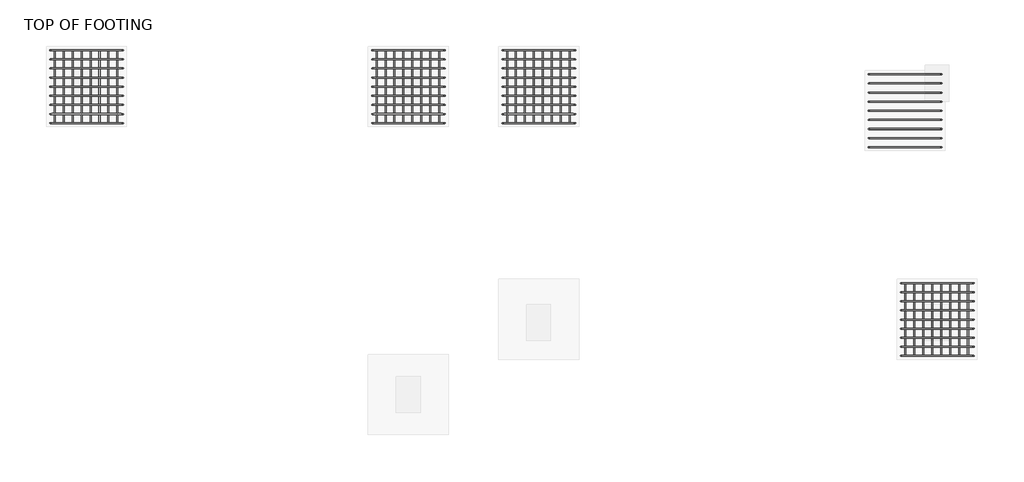
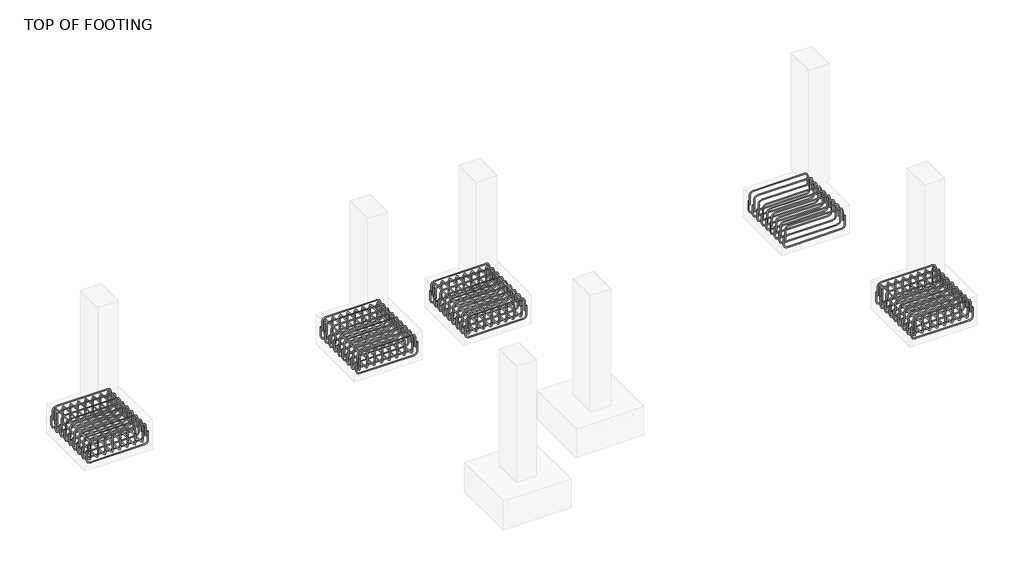
# One storey, part 19 of 20: 18 reinforcing bars.
"""IFC4 building model written with IfcOpenShell, lengths in millimetres."""

from ifc_helpers import new_model, si_unit, point, frame, origin, place, context, project, spatial, polyline, circle_curve, trimmed, segment, composite_curve, source, transform, mapped, element, save
from ifc_brep_helpers import swept_disk

model = new_model("IFC4")

# Units and contexts
model_context = context("Model", 3, world=origin())
ifc_project = project(units=[si_unit("LENGTHUNIT", "METRE", prefix="MILLI")], contexts=[model_context])

# Site, building, storey
site = spatial("IfcSite", under=ifc_project)
building = spatial("IfcBuilding", under=site)
storey = spatial("IfcBuildingStorey", under=building, Name="TOP OF FOOTING", Elevation=-1828.8)

# Reinforcing bars
placement = place(None, origin())
reinforcing_bar_shape = source(origin(), model_context, "Body", "SolidModel", [
    swept_disk(composite_curve([segment(polyline([(2628.3796816, 22141.4849362, -2006.6587682), (2628.3796816, 22141.4849362, -2153.9587682)]), True, "CONTINUOUS"), segment(trimmed(circle_curve(frame((2582.0296816, 22141.4849362, -2153.9587682), z_axis=(0.0, 1.0, 0.0), x_axis=(46.34999999999991, 0.0, 0.0)), 46.35), [point((2628.3796816, 22141.4849362, -2153.9587682))], [point((2582.0296816, 22141.4849362, -2200.3087682))], True, "CARTESIAN"), True, "CONTINUOUS"), segment(polyline([(2582.0296816, 22141.4849362, -2200.3087682), (1767.4296816, 22141.4849362, -2200.3087682)]), True, "CONTINUOUS"), segment(trimmed(circle_curve(frame((1767.4296816, 22141.4849362, -2153.9587682), z_axis=(0.0, 1.0, 0.0), x_axis=(0.0, 0.0, -46.34999999999991)), 46.35), [point((1767.4296816, 22141.4849362, -2200.3087682))], [point((1721.0796816, 22141.4849362, -2153.9587682))], True, "CARTESIAN"), True, "CONTINUOUS"), segment(polyline([(1721.0796816, 22141.4849362, -2153.9587682), (1721.0796816, 22141.4849362, -2006.6587682)]), True, "CONTINUOUS")], self_intersect=False), 6.35),
])
element("IfcReinforcingBar", 1, at=placement, inside=storey, context=model_context, shape_type="MappedRepresentation", body=[
    mapped(reinforcing_bar_shape, transform((0.0, 0.0, 0.0), x_axis=(1.0, 0.0, 0.0), y_axis=(0.0, 1.0, 0.0), z_axis=(0.0, 0.0, 1.0))),
    mapped(reinforcing_bar_shape, transform((0.0, -113.4125, 0.0), x_axis=(1.0, 0.0, 0.0), y_axis=(0.0, 1.0, 0.0), z_axis=(0.0, 0.0, 1.0))),
    mapped(reinforcing_bar_shape, transform((0.0, -226.825, 0.0), x_axis=(1.0, 0.0, 0.0), y_axis=(0.0, 1.0, 0.0), z_axis=(0.0, 0.0, 1.0))),
    mapped(reinforcing_bar_shape, transform((0.0, -340.2375, 0.0), x_axis=(1.0, 0.0, 0.0), y_axis=(0.0, 1.0, 0.0), z_axis=(0.0, 0.0, 1.0))),
    mapped(reinforcing_bar_shape, transform((0.0, -453.65, 0.0), x_axis=(1.0, 0.0, 0.0), y_axis=(0.0, 1.0, 0.0), z_axis=(0.0, 0.0, 1.0))),
    mapped(reinforcing_bar_shape, transform((0.0, -567.0625, 0.0), x_axis=(1.0, 0.0, 0.0), y_axis=(0.0, 1.0, 0.0), z_axis=(0.0, 0.0, 1.0))),
    mapped(reinforcing_bar_shape, transform((0.0, -680.475, 0.0), x_axis=(1.0, 0.0, 0.0), y_axis=(0.0, 1.0, 0.0), z_axis=(0.0, 0.0, 1.0))),
    mapped(reinforcing_bar_shape, transform((0.0, -793.8875, 0.0), x_axis=(1.0, 0.0, 0.0), y_axis=(0.0, 1.0, 0.0), z_axis=(0.0, 0.0, 1.0))),
    mapped(reinforcing_bar_shape, transform((0.0, -907.3, 0.0), x_axis=(1.0, 0.0, 0.0), y_axis=(0.0, 1.0, 0.0), z_axis=(0.0, 0.0, 1.0))),
])
reinforcing_bar_2_shape = source(origin(), model_context, "Body", "SolidModel", [
    swept_disk(composite_curve([segment(polyline([(1740.553793, 22141.4849362, -2068.8), (1740.553793, 22141.4849362, -1921.5)]), True, "CONTINUOUS"), segment(trimmed(circle_curve(frame((1786.903793, 22141.4849362, -1921.5), z_axis=(0.0, 1.0, 0.0), x_axis=(-46.34999999999991, 0.0, 0.0)), 46.35), [point((1740.553793, 22141.4849362, -1921.5))], [point((1786.903793, 22141.4849362, -1875.15))], True, "CARTESIAN"), True, "CONTINUOUS"), segment(polyline([(1786.903793, 22141.4849362, -1875.15), (2556.3671926, 22141.4849362, -1875.15)]), True, "CONTINUOUS"), segment(trimmed(circle_curve(frame((2556.3671926, 22141.4849362, -1921.5), z_axis=(0.0, 1.0, 0.0), x_axis=(0.0, 0.0, 46.34999999999991)), 46.35), [point((2556.3671926, 22141.4849362, -1875.15))], [point((2602.7171926, 22141.4849362, -1921.5))], True, "CARTESIAN"), True, "CONTINUOUS"), segment(polyline([(2602.7171926, 22141.4849362, -1921.5), (2602.7171926, 22141.4849362, -2068.8)]), True, "CONTINUOUS")], self_intersect=False), 6.35),
])
element("IfcReinforcingBar", 2, at=placement, inside=storey, context=model_context, shape_type="MappedRepresentation", body=[
    mapped(reinforcing_bar_2_shape, transform((0.0, 0.0, 0.0), x_axis=(1.0, 0.0, 0.0), y_axis=(0.0, 1.0, 0.0), z_axis=(0.0, 0.0, 1.0))),
    mapped(reinforcing_bar_2_shape, transform((0.0, -113.4125, 0.0), x_axis=(1.0, 0.0, 0.0), y_axis=(0.0, 1.0, 0.0), z_axis=(0.0, 0.0, 1.0))),
    mapped(reinforcing_bar_2_shape, transform((0.0, -226.825, 0.0), x_axis=(1.0, 0.0, 0.0), y_axis=(0.0, 1.0, 0.0), z_axis=(0.0, 0.0, 1.0))),
    mapped(reinforcing_bar_2_shape, transform((0.0, -340.2375, 0.0), x_axis=(1.0, 0.0, 0.0), y_axis=(0.0, 1.0, 0.0), z_axis=(0.0, 0.0, 1.0))),
    mapped(reinforcing_bar_2_shape, transform((0.0, -453.65, 0.0), x_axis=(1.0, 0.0, 0.0), y_axis=(0.0, 1.0, 0.0), z_axis=(0.0, 0.0, 1.0))),
    mapped(reinforcing_bar_2_shape, transform((0.0, -567.0625, 0.0), x_axis=(1.0, 0.0, 0.0), y_axis=(0.0, 1.0, 0.0), z_axis=(0.0, 0.0, 1.0))),
    mapped(reinforcing_bar_2_shape, transform((0.0, -680.475, 0.0), x_axis=(1.0, 0.0, 0.0), y_axis=(0.0, 1.0, 0.0), z_axis=(0.0, 0.0, 1.0))),
    mapped(reinforcing_bar_2_shape, transform((0.0, -793.8875, 0.0), x_axis=(1.0, 0.0, 0.0), y_axis=(0.0, 1.0, 0.0), z_axis=(0.0, 0.0, 1.0))),
    mapped(reinforcing_bar_2_shape, transform((0.0, -907.3, 0.0), x_axis=(1.0, 0.0, 0.0), y_axis=(0.0, 1.0, 0.0), z_axis=(0.0, 0.0, 1.0))),
])
reinforcing_bar_3_shape = source(origin(), model_context, "Body", "SolidModel", [
    swept_disk(composite_curve([segment(polyline([(2556.8827202, 22141.4849362, -2086.1951968), (2556.8827202, 22141.4849362, -1938.8951968)]), True, "CONTINUOUS"), segment(trimmed(circle_curve(frame((2556.8827202, 22095.1349362, -1938.8951968), z_axis=(1.0, 0.0, 0.0), x_axis=(0.0, 46.349999999998545, 0.0)), 46.35), [point((2556.8827202, 22141.4849362, -1938.8951968))], [point((2556.8827202, 22095.1349362, -1892.5451968))], True, "CARTESIAN"), True, "CONTINUOUS"), segment(polyline([(2556.8827202, 22095.1349362, -1892.5451968), (2556.8827202, 21280.5349362, -1892.5451968)]), True, "CONTINUOUS"), segment(trimmed(circle_curve(frame((2556.8827202, 21280.5349362, -1938.8951968), z_axis=(1.0, 0.0, 0.0), x_axis=(0.0, 0.0, 46.34999999999991)), 46.35), [point((2556.8827202, 21280.5349362, -1892.5451968))], [point((2556.8827202, 21234.1849362, -1938.8951968))], True, "CARTESIAN"), True, "CONTINUOUS"), segment(polyline([(2556.8827202, 21234.1849362, -1938.8951968), (2556.8827202, 21234.1849362, -2086.1951968)]), True, "CONTINUOUS")], self_intersect=False), 6.35),
])
element("IfcReinforcingBar", 3, at=placement, inside=storey, context=model_context, shape_type="MappedRepresentation", body=[
    mapped(reinforcing_bar_3_shape, transform((0.0, 0.0, 0.0), x_axis=(1.0, 0.0, 0.0), y_axis=(0.0, 1.0, 0.0), z_axis=(0.0, 0.0, 1.0))),
    mapped(reinforcing_bar_3_shape, transform((-111.2862402, 0.0, 0.0), x_axis=(1.0, 0.0, 0.0), y_axis=(0.0, 1.0, 0.0), z_axis=(0.0, 0.0, 1.0))),
    mapped(reinforcing_bar_3_shape, transform((-222.5724804, 0.0, 0.0), x_axis=(1.0, 0.0, 0.0), y_axis=(0.0, 1.0, 0.0), z_axis=(0.0, 0.0, 1.0))),
    mapped(reinforcing_bar_3_shape, transform((-333.8587205, 0.0, 0.0), x_axis=(1.0, 0.0, 0.0), y_axis=(0.0, 1.0, 0.0), z_axis=(0.0, 0.0, 1.0))),
    mapped(reinforcing_bar_3_shape, transform((-445.1449607, 0.0, 0.0), x_axis=(1.0, 0.0, 0.0), y_axis=(0.0, 1.0, 0.0), z_axis=(0.0, 0.0, 1.0))),
    mapped(reinforcing_bar_3_shape, transform((-556.4312009, 0.0, 0.0), x_axis=(1.0, 0.0, 0.0), y_axis=(0.0, 1.0, 0.0), z_axis=(0.0, 0.0, 1.0))),
    mapped(reinforcing_bar_3_shape, transform((-667.7174411, 0.0, 0.0), x_axis=(1.0, 0.0, 0.0), y_axis=(0.0, 1.0, 0.0), z_axis=(0.0, 0.0, 1.0))),
    mapped(reinforcing_bar_3_shape, transform((-779.0036813, 0.0, 0.0), x_axis=(1.0, 0.0, 0.0), y_axis=(0.0, 1.0, 0.0), z_axis=(0.0, 0.0, 1.0))),
])
reinforcing_bar_4_shape = source(origin(), model_context, "Body", "SolidModel", [
    swept_disk(composite_curve([segment(polyline([(1777.879039, 22141.4849362, -1979.1645013), (1777.879039, 22141.4849362, -2126.4645013)]), True, "CONTINUOUS"), segment(trimmed(circle_curve(frame((1777.879039, 22095.1349362, -2126.4645013), z_axis=(-1.0, 0.0, 0.0), x_axis=(0.0, 46.349999999998545, 0.0)), 46.35), [point((1777.879039, 22141.4849362, -2126.4645013))], [point((1777.879039, 22095.1349362, -2172.8145013))], True, "CARTESIAN"), True, "CONTINUOUS"), segment(polyline([(1777.879039, 22095.1349362, -2172.8145013), (1777.879039, 21280.5349362, -2172.8145013)]), True, "CONTINUOUS"), segment(trimmed(circle_curve(frame((1777.879039, 21280.5349362, -2126.4645013), z_axis=(-1.0, 0.0, 0.0), x_axis=(0.0, 0.0, -46.34999999999991)), 46.35), [point((1777.879039, 21280.5349362, -2172.8145013))], [point((1777.879039, 21234.1849362, -2126.4645013))], True, "CARTESIAN"), True, "CONTINUOUS"), segment(polyline([(1777.879039, 21234.1849362, -2126.4645013), (1777.879039, 21234.1849362, -1979.1645013)]), True, "CONTINUOUS")], self_intersect=False), 6.35),
])
element("IfcReinforcingBar", 4, at=placement, inside=storey, context=model_context, shape_type="MappedRepresentation", body=[
    mapped(reinforcing_bar_4_shape, transform((0.0, 0.0, 0.0), x_axis=(1.0, 0.0, 0.0), y_axis=(0.0, 1.0, 0.0), z_axis=(0.0, 0.0, 1.0))),
    mapped(reinforcing_bar_4_shape, transform((111.2862402, 0.0, 0.0), x_axis=(1.0, 0.0, 0.0), y_axis=(0.0, 1.0, 0.0), z_axis=(0.0, 0.0, 1.0))),
    mapped(reinforcing_bar_4_shape, transform((222.5724804, 0.0, 0.0), x_axis=(1.0, 0.0, 0.0), y_axis=(0.0, 1.0, 0.0), z_axis=(0.0, 0.0, 1.0))),
    mapped(reinforcing_bar_4_shape, transform((333.8587205, 0.0, 0.0), x_axis=(1.0, 0.0, 0.0), y_axis=(0.0, 1.0, 0.0), z_axis=(0.0, 0.0, 1.0))),
    mapped(reinforcing_bar_4_shape, transform((445.1449607, 0.0, 0.0), x_axis=(1.0, 0.0, 0.0), y_axis=(0.0, 1.0, 0.0), z_axis=(0.0, 0.0, 1.0))),
    mapped(reinforcing_bar_4_shape, transform((556.4312009, 0.0, 0.0), x_axis=(1.0, 0.0, 0.0), y_axis=(0.0, 1.0, 0.0), z_axis=(0.0, 0.0, 1.0))),
    mapped(reinforcing_bar_4_shape, transform((667.7174411, 0.0, 0.0), x_axis=(1.0, 0.0, 0.0), y_axis=(0.0, 1.0, 0.0), z_axis=(0.0, 0.0, 1.0))),
    mapped(reinforcing_bar_4_shape, transform((779.0036813, 0.0, 0.0), x_axis=(1.0, 0.0, 0.0), y_axis=(0.0, 1.0, 0.0), z_axis=(0.0, 0.0, 1.0))),
])
reinforcing_bar_5_shape = source(origin(), model_context, "Body", "SolidModel", [
    swept_disk(composite_curve([segment(polyline([(6636.1748054, 22141.4849362, -2006.6587682), (6636.1748054, 22141.4849362, -2153.9587682)]), True, "CONTINUOUS"), segment(trimmed(circle_curve(frame((6589.8248054, 22141.4849362, -2153.9587682), z_axis=(0.0, 1.0, 0.0), x_axis=(46.350000000000364, 0.0, 0.0)), 46.35), [point((6636.1748054, 22141.4849362, -2153.9587682))], [point((6589.8248054, 22141.4849362, -2200.3087682))], True, "CARTESIAN"), True, "CONTINUOUS"), segment(polyline([(6589.8248054, 22141.4849362, -2200.3087682), (5775.2248054, 22141.4849362, -2200.3087682)]), True, "CONTINUOUS"), segment(trimmed(circle_curve(frame((5775.2248054, 22141.4849362, -2153.9587682), z_axis=(0.0, 1.0, 0.0), x_axis=(0.0, 0.0, -46.34999999999991)), 46.35), [point((5775.2248054, 22141.4849362, -2200.3087682))], [point((5728.8748054, 22141.4849362, -2153.9587682))], True, "CARTESIAN"), True, "CONTINUOUS"), segment(polyline([(5728.8748054, 22141.4849362, -2153.9587682), (5728.8748054, 22141.4849362, -2006.6587682)]), True, "CONTINUOUS")], self_intersect=False), 6.35),
])
element("IfcReinforcingBar", 5, at=placement, inside=storey, context=model_context, shape_type="MappedRepresentation", body=[
    mapped(reinforcing_bar_5_shape, transform((0.0, 0.0, 0.0), x_axis=(1.0, 0.0, 0.0), y_axis=(0.0, 1.0, 0.0), z_axis=(0.0, 0.0, 1.0))),
    mapped(reinforcing_bar_5_shape, transform((0.0, -113.4125, 0.0), x_axis=(1.0, 0.0, 0.0), y_axis=(0.0, 1.0, 0.0), z_axis=(0.0, 0.0, 1.0))),
    mapped(reinforcing_bar_5_shape, transform((0.0, -226.825, 0.0), x_axis=(1.0, 0.0, 0.0), y_axis=(0.0, 1.0, 0.0), z_axis=(0.0, 0.0, 1.0))),
    mapped(reinforcing_bar_5_shape, transform((0.0, -340.2375, 0.0), x_axis=(1.0, 0.0, 0.0), y_axis=(0.0, 1.0, 0.0), z_axis=(0.0, 0.0, 1.0))),
    mapped(reinforcing_bar_5_shape, transform((0.0, -453.65, 0.0), x_axis=(1.0, 0.0, 0.0), y_axis=(0.0, 1.0, 0.0), z_axis=(0.0, 0.0, 1.0))),
    mapped(reinforcing_bar_5_shape, transform((0.0, -567.0625, 0.0), x_axis=(1.0, 0.0, 0.0), y_axis=(0.0, 1.0, 0.0), z_axis=(0.0, 0.0, 1.0))),
    mapped(reinforcing_bar_5_shape, transform((0.0, -680.475, 0.0), x_axis=(1.0, 0.0, 0.0), y_axis=(0.0, 1.0, 0.0), z_axis=(0.0, 0.0, 1.0))),
    mapped(reinforcing_bar_5_shape, transform((0.0, -793.8875, 0.0), x_axis=(1.0, 0.0, 0.0), y_axis=(0.0, 1.0, 0.0), z_axis=(0.0, 0.0, 1.0))),
    mapped(reinforcing_bar_5_shape, transform((0.0, -907.3, 0.0), x_axis=(1.0, 0.0, 0.0), y_axis=(0.0, 1.0, 0.0), z_axis=(0.0, 0.0, 1.0))),
])
reinforcing_bar_6_shape = source(origin(), model_context, "Body", "SolidModel", [
    swept_disk(composite_curve([segment(polyline([(5748.3489167, 22141.4849362, -2068.8), (5748.3489167, 22141.4849362, -1921.5)]), True, "CONTINUOUS"), segment(trimmed(circle_curve(frame((5794.6989167, 22141.4849362, -1921.5), z_axis=(0.0, 1.0, 0.0), x_axis=(-46.350000000000364, 0.0, 0.0)), 46.35), [point((5748.3489167, 22141.4849362, -1921.5))], [point((5794.6989167, 22141.4849362, -1875.15))], True, "CARTESIAN"), True, "CONTINUOUS"), segment(polyline([(5794.6989167, 22141.4849362, -1875.15), (6564.1623164, 22141.4849362, -1875.15)]), True, "CONTINUOUS"), segment(trimmed(circle_curve(frame((6564.1623164, 22141.4849362, -1921.5), z_axis=(0.0, 1.0, 0.0), x_axis=(0.0, 0.0, 46.34999999999991)), 46.35), [point((6564.1623164, 22141.4849362, -1875.15))], [point((6610.5123164, 22141.4849362, -1921.5))], True, "CARTESIAN"), True, "CONTINUOUS"), segment(polyline([(6610.5123164, 22141.4849362, -1921.5), (6610.5123164, 22141.4849362, -2068.8)]), True, "CONTINUOUS")], self_intersect=False), 6.35),
])
element("IfcReinforcingBar", 6, at=placement, inside=storey, context=model_context, shape_type="MappedRepresentation", body=[
    mapped(reinforcing_bar_6_shape, transform((0.0, 0.0, 0.0), x_axis=(1.0, 0.0, 0.0), y_axis=(0.0, 1.0, 0.0), z_axis=(0.0, 0.0, 1.0))),
    mapped(reinforcing_bar_6_shape, transform((0.0, -113.4125, 0.0), x_axis=(1.0, 0.0, 0.0), y_axis=(0.0, 1.0, 0.0), z_axis=(0.0, 0.0, 1.0))),
    mapped(reinforcing_bar_6_shape, transform((0.0, -226.825, 0.0), x_axis=(1.0, 0.0, 0.0), y_axis=(0.0, 1.0, 0.0), z_axis=(0.0, 0.0, 1.0))),
    mapped(reinforcing_bar_6_shape, transform((0.0, -340.2375, 0.0), x_axis=(1.0, 0.0, 0.0), y_axis=(0.0, 1.0, 0.0), z_axis=(0.0, 0.0, 1.0))),
    mapped(reinforcing_bar_6_shape, transform((0.0, -453.65, 0.0), x_axis=(1.0, 0.0, 0.0), y_axis=(0.0, 1.0, 0.0), z_axis=(0.0, 0.0, 1.0))),
    mapped(reinforcing_bar_6_shape, transform((0.0, -567.0625, 0.0), x_axis=(1.0, 0.0, 0.0), y_axis=(0.0, 1.0, 0.0), z_axis=(0.0, 0.0, 1.0))),
    mapped(reinforcing_bar_6_shape, transform((0.0, -680.475, 0.0), x_axis=(1.0, 0.0, 0.0), y_axis=(0.0, 1.0, 0.0), z_axis=(0.0, 0.0, 1.0))),
    mapped(reinforcing_bar_6_shape, transform((0.0, -793.8875, 0.0), x_axis=(1.0, 0.0, 0.0), y_axis=(0.0, 1.0, 0.0), z_axis=(0.0, 0.0, 1.0))),
    mapped(reinforcing_bar_6_shape, transform((0.0, -907.3, 0.0), x_axis=(1.0, 0.0, 0.0), y_axis=(0.0, 1.0, 0.0), z_axis=(0.0, 0.0, 1.0))),
])
reinforcing_bar_7_shape = source(origin(), model_context, "Body", "SolidModel", [
    swept_disk(composite_curve([segment(polyline([(6564.677844, 22141.4849362, -2086.1951968), (6564.677844, 22141.4849362, -1938.8951968)]), True, "CONTINUOUS"), segment(trimmed(circle_curve(frame((6564.677844, 22095.1349362, -1938.8951968), z_axis=(1.0, 0.0, 0.0), x_axis=(0.0, 46.349999999998545, 0.0)), 46.35), [point((6564.677844, 22141.4849362, -1938.8951968))], [point((6564.677844, 22095.1349362, -1892.5451968))], True, "CARTESIAN"), True, "CONTINUOUS"), segment(polyline([(6564.677844, 22095.1349362, -1892.5451968), (6564.677844, 21280.5349362, -1892.5451968)]), True, "CONTINUOUS"), segment(trimmed(circle_curve(frame((6564.677844, 21280.5349362, -1938.8951968), z_axis=(1.0, 0.0, 0.0), x_axis=(0.0, 0.0, 46.34999999999991)), 46.35), [point((6564.677844, 21280.5349362, -1892.5451968))], [point((6564.677844, 21234.1849362, -1938.8951968))], True, "CARTESIAN"), True, "CONTINUOUS"), segment(polyline([(6564.677844, 21234.1849362, -1938.8951968), (6564.677844, 21234.1849362, -2086.1951968)]), True, "CONTINUOUS")], self_intersect=False), 6.35),
])
element("IfcReinforcingBar", 7, at=placement, inside=storey, context=model_context, shape_type="MappedRepresentation", body=[
    mapped(reinforcing_bar_7_shape, transform((0.0, 0.0, 0.0), x_axis=(1.0, 0.0, 0.0), y_axis=(0.0, 1.0, 0.0), z_axis=(0.0, 0.0, 1.0))),
    mapped(reinforcing_bar_7_shape, transform((-111.2862402, 0.0, 0.0), x_axis=(1.0, 0.0, 0.0), y_axis=(0.0, 1.0, 0.0), z_axis=(0.0, 0.0, 1.0))),
    mapped(reinforcing_bar_7_shape, transform((-222.5724804, 0.0, 0.0), x_axis=(1.0, 0.0, 0.0), y_axis=(0.0, 1.0, 0.0), z_axis=(0.0, 0.0, 1.0))),
    mapped(reinforcing_bar_7_shape, transform((-333.8587205, 0.0, 0.0), x_axis=(1.0, 0.0, 0.0), y_axis=(0.0, 1.0, 0.0), z_axis=(0.0, 0.0, 1.0))),
    mapped(reinforcing_bar_7_shape, transform((-445.1449607, 0.0, 0.0), x_axis=(1.0, 0.0, 0.0), y_axis=(0.0, 1.0, 0.0), z_axis=(0.0, 0.0, 1.0))),
    mapped(reinforcing_bar_7_shape, transform((-556.4312009, 0.0, 0.0), x_axis=(1.0, 0.0, 0.0), y_axis=(0.0, 1.0, 0.0), z_axis=(0.0, 0.0, 1.0))),
    mapped(reinforcing_bar_7_shape, transform((-667.7174411, 0.0, 0.0), x_axis=(1.0, 0.0, 0.0), y_axis=(0.0, 1.0, 0.0), z_axis=(0.0, 0.0, 1.0))),
    mapped(reinforcing_bar_7_shape, transform((-779.0036813, 0.0, 0.0), x_axis=(1.0, 0.0, 0.0), y_axis=(0.0, 1.0, 0.0), z_axis=(0.0, 0.0, 1.0))),
])
reinforcing_bar_8_shape = source(origin(), model_context, "Body", "SolidModel", [
    swept_disk(composite_curve([segment(polyline([(5785.6741627, 22141.4849362, -1979.1645013), (5785.6741627, 22141.4849362, -2126.4645013)]), True, "CONTINUOUS"), segment(trimmed(circle_curve(frame((5785.6741627, 22095.1349362, -2126.4645013), z_axis=(-1.0, 0.0, 0.0), x_axis=(0.0, 46.349999999998545, 0.0)), 46.35), [point((5785.6741627, 22141.4849362, -2126.4645013))], [point((5785.6741627, 22095.1349362, -2172.8145013))], True, "CARTESIAN"), True, "CONTINUOUS"), segment(polyline([(5785.6741627, 22095.1349362, -2172.8145013), (5785.6741627, 21280.5349362, -2172.8145013)]), True, "CONTINUOUS"), segment(trimmed(circle_curve(frame((5785.6741627, 21280.5349362, -2126.4645013), z_axis=(-1.0, 0.0, 0.0), x_axis=(0.0, 0.0, -46.34999999999991)), 46.35), [point((5785.6741627, 21280.5349362, -2172.8145013))], [point((5785.6741627, 21234.1849362, -2126.4645013))], True, "CARTESIAN"), True, "CONTINUOUS"), segment(polyline([(5785.6741627, 21234.1849362, -2126.4645013), (5785.6741627, 21234.1849362, -1979.1645013)]), True, "CONTINUOUS")], self_intersect=False), 6.35),
])
element("IfcReinforcingBar", 8, at=placement, inside=storey, context=model_context, shape_type="MappedRepresentation", body=[
    mapped(reinforcing_bar_8_shape, transform((0.0, 0.0, 0.0), x_axis=(1.0, 0.0, 0.0), y_axis=(0.0, 1.0, 0.0), z_axis=(0.0, 0.0, 1.0))),
    mapped(reinforcing_bar_8_shape, transform((111.2862402, 0.0, 0.0), x_axis=(1.0, 0.0, 0.0), y_axis=(0.0, 1.0, 0.0), z_axis=(0.0, 0.0, 1.0))),
    mapped(reinforcing_bar_8_shape, transform((222.5724804, 0.0, 0.0), x_axis=(1.0, 0.0, 0.0), y_axis=(0.0, 1.0, 0.0), z_axis=(0.0, 0.0, 1.0))),
    mapped(reinforcing_bar_8_shape, transform((333.8587205, 0.0, 0.0), x_axis=(1.0, 0.0, 0.0), y_axis=(0.0, 1.0, 0.0), z_axis=(0.0, 0.0, 1.0))),
    mapped(reinforcing_bar_8_shape, transform((445.1449607, 0.0, 0.0), x_axis=(1.0, 0.0, 0.0), y_axis=(0.0, 1.0, 0.0), z_axis=(0.0, 0.0, 1.0))),
    mapped(reinforcing_bar_8_shape, transform((556.4312009, 0.0, 0.0), x_axis=(1.0, 0.0, 0.0), y_axis=(0.0, 1.0, 0.0), z_axis=(0.0, 0.0, 1.0))),
    mapped(reinforcing_bar_8_shape, transform((667.7174411, 0.0, 0.0), x_axis=(1.0, 0.0, 0.0), y_axis=(0.0, 1.0, 0.0), z_axis=(0.0, 0.0, 1.0))),
    mapped(reinforcing_bar_8_shape, transform((779.0036813, 0.0, 0.0), x_axis=(1.0, 0.0, 0.0), y_axis=(0.0, 1.0, 0.0), z_axis=(0.0, 0.0, 1.0))),
])
reinforcing_bar_9_shape = source(origin(), model_context, "Body", "SolidModel", [
    swept_disk(composite_curve([segment(polyline([(8260.5179014, 22141.4849362, -2006.6587682), (8260.5179014, 22141.4849362, -2153.9587682)]), True, "CONTINUOUS"), segment(trimmed(circle_curve(frame((8214.1679014, 22141.4849362, -2153.9587682), z_axis=(0.0, 1.0, 0.0), x_axis=(46.350000000000364, 0.0, 0.0)), 46.35), [point((8260.5179014, 22141.4849362, -2153.9587682))], [point((8214.1679014, 22141.4849362, -2200.3087682))], True, "CARTESIAN"), True, "CONTINUOUS"), segment(polyline([(8214.1679014, 22141.4849362, -2200.3087682), (7399.5679014, 22141.4849362, -2200.3087682)]), True, "CONTINUOUS"), segment(trimmed(circle_curve(frame((7399.5679014, 22141.4849362, -2153.9587682), z_axis=(0.0, 1.0, 0.0), x_axis=(0.0, 0.0, -46.34999999999991)), 46.35), [point((7399.5679014, 22141.4849362, -2200.3087682))], [point((7353.2179014, 22141.4849362, -2153.9587682))], True, "CARTESIAN"), True, "CONTINUOUS"), segment(polyline([(7353.2179014, 22141.4849362, -2153.9587682), (7353.2179014, 22141.4849362, -2006.6587682)]), True, "CONTINUOUS")], self_intersect=False), 6.35),
])
element("IfcReinforcingBar", 9, at=placement, inside=storey, context=model_context, shape_type="MappedRepresentation", body=[
    mapped(reinforcing_bar_9_shape, transform((0.0, 0.0, 0.0), x_axis=(1.0, 0.0, 0.0), y_axis=(0.0, 1.0, 0.0), z_axis=(0.0, 0.0, 1.0))),
    mapped(reinforcing_bar_9_shape, transform((0.0, -113.4125, 0.0), x_axis=(1.0, 0.0, 0.0), y_axis=(0.0, 1.0, 0.0), z_axis=(0.0, 0.0, 1.0))),
    mapped(reinforcing_bar_9_shape, transform((0.0, -226.825, 0.0), x_axis=(1.0, 0.0, 0.0), y_axis=(0.0, 1.0, 0.0), z_axis=(0.0, 0.0, 1.0))),
    mapped(reinforcing_bar_9_shape, transform((0.0, -340.2375, 0.0), x_axis=(1.0, 0.0, 0.0), y_axis=(0.0, 1.0, 0.0), z_axis=(0.0, 0.0, 1.0))),
    mapped(reinforcing_bar_9_shape, transform((0.0, -453.65, 0.0), x_axis=(1.0, 0.0, 0.0), y_axis=(0.0, 1.0, 0.0), z_axis=(0.0, 0.0, 1.0))),
    mapped(reinforcing_bar_9_shape, transform((0.0, -567.0625, 0.0), x_axis=(1.0, 0.0, 0.0), y_axis=(0.0, 1.0, 0.0), z_axis=(0.0, 0.0, 1.0))),
    mapped(reinforcing_bar_9_shape, transform((0.0, -680.475, 0.0), x_axis=(1.0, 0.0, 0.0), y_axis=(0.0, 1.0, 0.0), z_axis=(0.0, 0.0, 1.0))),
    mapped(reinforcing_bar_9_shape, transform((0.0, -793.8875, 0.0), x_axis=(1.0, 0.0, 0.0), y_axis=(0.0, 1.0, 0.0), z_axis=(0.0, 0.0, 1.0))),
    mapped(reinforcing_bar_9_shape, transform((0.0, -907.3, 0.0), x_axis=(1.0, 0.0, 0.0), y_axis=(0.0, 1.0, 0.0), z_axis=(0.0, 0.0, 1.0))),
])
reinforcing_bar_10_shape = source(origin(), model_context, "Body", "SolidModel", [
    swept_disk(composite_curve([segment(polyline([(7372.6920127, 22141.4849362, -2068.8), (7372.6920127, 22141.4849362, -1921.5)]), True, "CONTINUOUS"), segment(trimmed(circle_curve(frame((7419.0420127, 22141.4849362, -1921.5), z_axis=(0.0, 1.0, 0.0), x_axis=(-46.349999999999454, 0.0, 0.0)), 46.35), [point((7372.6920127, 22141.4849362, -1921.5))], [point((7419.0420127, 22141.4849362, -1875.15))], True, "CARTESIAN"), True, "CONTINUOUS"), segment(polyline([(7419.0420127, 22141.4849362, -1875.15), (8188.5054124, 22141.4849362, -1875.15)]), True, "CONTINUOUS"), segment(trimmed(circle_curve(frame((8188.5054124, 22141.4849362, -1921.5), z_axis=(0.0, 1.0, 0.0), x_axis=(0.0, 0.0, 46.34999999999991)), 46.35), [point((8188.5054124, 22141.4849362, -1875.15))], [point((8234.8554124, 22141.4849362, -1921.5))], True, "CARTESIAN"), True, "CONTINUOUS"), segment(polyline([(8234.8554124, 22141.4849362, -1921.5), (8234.8554124, 22141.4849362, -2068.8)]), True, "CONTINUOUS")], self_intersect=False), 6.35),
])
element("IfcReinforcingBar", 10, at=placement, inside=storey, context=model_context, shape_type="MappedRepresentation", body=[
    mapped(reinforcing_bar_10_shape, transform((0.0, 0.0, 0.0), x_axis=(1.0, 0.0, 0.0), y_axis=(0.0, 1.0, 0.0), z_axis=(0.0, 0.0, 1.0))),
    mapped(reinforcing_bar_10_shape, transform((0.0, -113.4125, 0.0), x_axis=(1.0, 0.0, 0.0), y_axis=(0.0, 1.0, 0.0), z_axis=(0.0, 0.0, 1.0))),
    mapped(reinforcing_bar_10_shape, transform((0.0, -226.825, 0.0), x_axis=(1.0, 0.0, 0.0), y_axis=(0.0, 1.0, 0.0), z_axis=(0.0, 0.0, 1.0))),
    mapped(reinforcing_bar_10_shape, transform((0.0, -340.2375, 0.0), x_axis=(1.0, 0.0, 0.0), y_axis=(0.0, 1.0, 0.0), z_axis=(0.0, 0.0, 1.0))),
    mapped(reinforcing_bar_10_shape, transform((0.0, -453.65, 0.0), x_axis=(1.0, 0.0, 0.0), y_axis=(0.0, 1.0, 0.0), z_axis=(0.0, 0.0, 1.0))),
    mapped(reinforcing_bar_10_shape, transform((0.0, -567.0625, 0.0), x_axis=(1.0, 0.0, 0.0), y_axis=(0.0, 1.0, 0.0), z_axis=(0.0, 0.0, 1.0))),
    mapped(reinforcing_bar_10_shape, transform((0.0, -680.475, 0.0), x_axis=(1.0, 0.0, 0.0), y_axis=(0.0, 1.0, 0.0), z_axis=(0.0, 0.0, 1.0))),
    mapped(reinforcing_bar_10_shape, transform((0.0, -793.8875, 0.0), x_axis=(1.0, 0.0, 0.0), y_axis=(0.0, 1.0, 0.0), z_axis=(0.0, 0.0, 1.0))),
    mapped(reinforcing_bar_10_shape, transform((0.0, -907.3, 0.0), x_axis=(1.0, 0.0, 0.0), y_axis=(0.0, 1.0, 0.0), z_axis=(0.0, 0.0, 1.0))),
])
reinforcing_bar_11_shape = source(origin(), model_context, "Body", "SolidModel", [
    swept_disk(composite_curve([segment(polyline([(8189.02094, 22141.4849362, -2086.1951968), (8189.02094, 22141.4849362, -1938.8951968)]), True, "CONTINUOUS"), segment(trimmed(circle_curve(frame((8189.02094, 22095.1349362, -1938.8951968), z_axis=(1.0, 0.0, 0.0), x_axis=(0.0, 46.349999999998545, 0.0)), 46.35), [point((8189.02094, 22141.4849362, -1938.8951968))], [point((8189.02094, 22095.1349362, -1892.5451968))], True, "CARTESIAN"), True, "CONTINUOUS"), segment(polyline([(8189.02094, 22095.1349362, -1892.5451968), (8189.02094, 21280.5349362, -1892.5451968)]), True, "CONTINUOUS"), segment(trimmed(circle_curve(frame((8189.02094, 21280.5349362, -1938.8951968), z_axis=(1.0, 0.0, 0.0), x_axis=(0.0, 0.0, 46.34999999999991)), 46.35), [point((8189.02094, 21280.5349362, -1892.5451968))], [point((8189.02094, 21234.1849362, -1938.8951968))], True, "CARTESIAN"), True, "CONTINUOUS"), segment(polyline([(8189.02094, 21234.1849362, -1938.8951968), (8189.02094, 21234.1849362, -2086.1951968)]), True, "CONTINUOUS")], self_intersect=False), 6.35),
])
element("IfcReinforcingBar", 11, at=placement, inside=storey, context=model_context, shape_type="MappedRepresentation", body=[
    mapped(reinforcing_bar_11_shape, transform((0.0, 0.0, 0.0), x_axis=(1.0, 0.0, 0.0), y_axis=(0.0, 1.0, 0.0), z_axis=(0.0, 0.0, 1.0))),
    mapped(reinforcing_bar_11_shape, transform((-111.2862402, 0.0, 0.0), x_axis=(1.0, 0.0, 0.0), y_axis=(0.0, 1.0, 0.0), z_axis=(0.0, 0.0, 1.0))),
    mapped(reinforcing_bar_11_shape, transform((-222.5724804, 0.0, 0.0), x_axis=(1.0, 0.0, 0.0), y_axis=(0.0, 1.0, 0.0), z_axis=(0.0, 0.0, 1.0))),
    mapped(reinforcing_bar_11_shape, transform((-333.8587205, 0.0, 0.0), x_axis=(1.0, 0.0, 0.0), y_axis=(0.0, 1.0, 0.0), z_axis=(0.0, 0.0, 1.0))),
    mapped(reinforcing_bar_11_shape, transform((-445.1449607, 0.0, 0.0), x_axis=(1.0, 0.0, 0.0), y_axis=(0.0, 1.0, 0.0), z_axis=(0.0, 0.0, 1.0))),
    mapped(reinforcing_bar_11_shape, transform((-556.4312009, 0.0, 0.0), x_axis=(1.0, 0.0, 0.0), y_axis=(0.0, 1.0, 0.0), z_axis=(0.0, 0.0, 1.0))),
    mapped(reinforcing_bar_11_shape, transform((-667.7174411, 0.0, 0.0), x_axis=(1.0, 0.0, 0.0), y_axis=(0.0, 1.0, 0.0), z_axis=(0.0, 0.0, 1.0))),
    mapped(reinforcing_bar_11_shape, transform((-779.0036813, 0.0, 0.0), x_axis=(1.0, 0.0, 0.0), y_axis=(0.0, 1.0, 0.0), z_axis=(0.0, 0.0, 1.0))),
])
reinforcing_bar_12_shape = source(origin(), model_context, "Body", "SolidModel", [
    swept_disk(composite_curve([segment(polyline([(7410.0172587, 22141.4849362, -1979.1645013), (7410.0172587, 22141.4849362, -2126.4645013)]), True, "CONTINUOUS"), segment(trimmed(circle_curve(frame((7410.0172587, 22095.1349362, -2126.4645013), z_axis=(-1.0, 0.0, 0.0), x_axis=(0.0, 46.349999999998545, 0.0)), 46.35), [point((7410.0172587, 22141.4849362, -2126.4645013))], [point((7410.0172587, 22095.1349362, -2172.8145013))], True, "CARTESIAN"), True, "CONTINUOUS"), segment(polyline([(7410.0172587, 22095.1349362, -2172.8145013), (7410.0172587, 21280.5349362, -2172.8145013)]), True, "CONTINUOUS"), segment(trimmed(circle_curve(frame((7410.0172587, 21280.5349362, -2126.4645013), z_axis=(-1.0, 0.0, 0.0), x_axis=(0.0, 0.0, -46.34999999999991)), 46.35), [point((7410.0172587, 21280.5349362, -2172.8145013))], [point((7410.0172587, 21234.1849362, -2126.4645013))], True, "CARTESIAN"), True, "CONTINUOUS"), segment(polyline([(7410.0172587, 21234.1849362, -2126.4645013), (7410.0172587, 21234.1849362, -1979.1645013)]), True, "CONTINUOUS")], self_intersect=False), 6.35),
])
element("IfcReinforcingBar", 12, at=placement, inside=storey, context=model_context, shape_type="MappedRepresentation", body=[
    mapped(reinforcing_bar_12_shape, transform((0.0, 0.0, 0.0), x_axis=(1.0, 0.0, 0.0), y_axis=(0.0, 1.0, 0.0), z_axis=(0.0, 0.0, 1.0))),
    mapped(reinforcing_bar_12_shape, transform((111.2862402, 0.0, 0.0), x_axis=(1.0, 0.0, 0.0), y_axis=(0.0, 1.0, 0.0), z_axis=(0.0, 0.0, 1.0))),
    mapped(reinforcing_bar_12_shape, transform((222.5724804, 0.0, 0.0), x_axis=(1.0, 0.0, 0.0), y_axis=(0.0, 1.0, 0.0), z_axis=(0.0, 0.0, 1.0))),
    mapped(reinforcing_bar_12_shape, transform((333.8587205, 0.0, 0.0), x_axis=(1.0, 0.0, 0.0), y_axis=(0.0, 1.0, 0.0), z_axis=(0.0, 0.0, 1.0))),
    mapped(reinforcing_bar_12_shape, transform((445.1449607, 0.0, 0.0), x_axis=(1.0, 0.0, 0.0), y_axis=(0.0, 1.0, 0.0), z_axis=(0.0, 0.0, 1.0))),
    mapped(reinforcing_bar_12_shape, transform((556.4312009, 0.0, 0.0), x_axis=(1.0, 0.0, 0.0), y_axis=(0.0, 1.0, 0.0), z_axis=(0.0, 0.0, 1.0))),
    mapped(reinforcing_bar_12_shape, transform((667.7174411, 0.0, 0.0), x_axis=(1.0, 0.0, 0.0), y_axis=(0.0, 1.0, 0.0), z_axis=(0.0, 0.0, 1.0))),
    mapped(reinforcing_bar_12_shape, transform((779.0036813, 0.0, 0.0), x_axis=(1.0, 0.0, 0.0), y_axis=(0.0, 1.0, 0.0), z_axis=(0.0, 0.0, 1.0))),
])
reinforcing_bar_13_shape = source(origin(), model_context, "Body", "SolidModel", [
    swept_disk(composite_curve([segment(polyline([(12822.7663908, 21841.4849362, -2006.6587682), (12822.7663908, 21841.4849362, -2153.9587682)]), True, "CONTINUOUS"), segment(trimmed(circle_curve(frame((12776.4163908, 21841.4849362, -2153.9587682), z_axis=(0.0, 1.0, 0.0), x_axis=(46.350000000000364, 0.0, 0.0)), 46.35), [point((12822.7663908, 21841.4849362, -2153.9587682))], [point((12776.4163908, 21841.4849362, -2200.3087682))], True, "CARTESIAN"), True, "CONTINUOUS"), segment(polyline([(12776.4163908, 21841.4849362, -2200.3087682), (11961.8163908, 21841.4849362, -2200.3087682)]), True, "CONTINUOUS"), segment(trimmed(circle_curve(frame((11961.8163908, 21841.4849362, -2153.9587682), z_axis=(0.0, 1.0, 0.0), x_axis=(0.0, 0.0, -46.34999999999991)), 46.35), [point((11961.8163908, 21841.4849362, -2200.3087682))], [point((11915.4663908, 21841.4849362, -2153.9587682))], True, "CARTESIAN"), True, "CONTINUOUS"), segment(polyline([(11915.4663908, 21841.4849362, -2153.9587682), (11915.4663908, 21841.4849362, -2006.6587682)]), True, "CONTINUOUS")], self_intersect=False), 6.35),
])
element("IfcReinforcingBar", 13, at=placement, inside=storey, context=model_context, shape_type="MappedRepresentation", body=[
    mapped(reinforcing_bar_13_shape, transform((0.0, 0.0, 0.0), x_axis=(1.0, 0.0, 0.0), y_axis=(0.0, 1.0, 0.0), z_axis=(0.0, 0.0, 1.0))),
    mapped(reinforcing_bar_13_shape, transform((0.0, -113.4125, 0.0), x_axis=(1.0, 0.0, 0.0), y_axis=(0.0, 1.0, 0.0), z_axis=(0.0, 0.0, 1.0))),
    mapped(reinforcing_bar_13_shape, transform((0.0, -226.825, 0.0), x_axis=(1.0, 0.0, 0.0), y_axis=(0.0, 1.0, 0.0), z_axis=(0.0, 0.0, 1.0))),
    mapped(reinforcing_bar_13_shape, transform((0.0, -340.2375, 0.0), x_axis=(1.0, 0.0, 0.0), y_axis=(0.0, 1.0, 0.0), z_axis=(0.0, 0.0, 1.0))),
    mapped(reinforcing_bar_13_shape, transform((0.0, -453.65, 0.0), x_axis=(1.0, 0.0, 0.0), y_axis=(0.0, 1.0, 0.0), z_axis=(0.0, 0.0, 1.0))),
    mapped(reinforcing_bar_13_shape, transform((0.0, -567.0625, 0.0), x_axis=(1.0, 0.0, 0.0), y_axis=(0.0, 1.0, 0.0), z_axis=(0.0, 0.0, 1.0))),
    mapped(reinforcing_bar_13_shape, transform((0.0, -680.475, 0.0), x_axis=(1.0, 0.0, 0.0), y_axis=(0.0, 1.0, 0.0), z_axis=(0.0, 0.0, 1.0))),
    mapped(reinforcing_bar_13_shape, transform((0.0, -793.8875, 0.0), x_axis=(1.0, 0.0, 0.0), y_axis=(0.0, 1.0, 0.0), z_axis=(0.0, 0.0, 1.0))),
    mapped(reinforcing_bar_13_shape, transform((0.0, -907.3, 0.0), x_axis=(1.0, 0.0, 0.0), y_axis=(0.0, 1.0, 0.0), z_axis=(0.0, 0.0, 1.0))),
])
reinforcing_bar_14_shape = source(origin(), model_context, "Body", "SolidModel", [
    swept_disk(composite_curve([segment(polyline([(11934.9405021, 21841.4849362, -2068.8), (11934.9405021, 21841.4849362, -1921.5)]), True, "CONTINUOUS"), segment(trimmed(circle_curve(frame((11981.2905021, 21841.4849362, -1921.5), z_axis=(0.0, 1.0, 0.0), x_axis=(-46.350000000000364, 0.0, 0.0)), 46.35), [point((11934.9405021, 21841.4849362, -1921.5))], [point((11981.2905021, 21841.4849362, -1875.15))], True, "CARTESIAN"), True, "CONTINUOUS"), segment(polyline([(11981.2905021, 21841.4849362, -1875.15), (12750.7539017, 21841.4849362, -1875.15)]), True, "CONTINUOUS"), segment(trimmed(circle_curve(frame((12750.7539017, 21841.4849362, -1921.5), z_axis=(0.0, 1.0, 0.0), x_axis=(0.0, 0.0, 46.34999999999991)), 46.35), [point((12750.7539017, 21841.4849362, -1875.15))], [point((12797.1039017, 21841.4849362, -1921.5))], True, "CARTESIAN"), True, "CONTINUOUS"), segment(polyline([(12797.1039017, 21841.4849362, -1921.5), (12797.1039017, 21841.4849362, -2068.8)]), True, "CONTINUOUS")], self_intersect=False), 6.35),
])
element("IfcReinforcingBar", 14, at=placement, inside=storey, context=model_context, shape_type="MappedRepresentation", body=[
    mapped(reinforcing_bar_14_shape, transform((0.0, 0.0, 0.0), x_axis=(1.0, 0.0, 0.0), y_axis=(0.0, 1.0, 0.0), z_axis=(0.0, 0.0, 1.0))),
    mapped(reinforcing_bar_14_shape, transform((0.0, -113.4125, 0.0), x_axis=(1.0, 0.0, 0.0), y_axis=(0.0, 1.0, 0.0), z_axis=(0.0, 0.0, 1.0))),
    mapped(reinforcing_bar_14_shape, transform((0.0, -226.825, 0.0), x_axis=(1.0, 0.0, 0.0), y_axis=(0.0, 1.0, 0.0), z_axis=(0.0, 0.0, 1.0))),
    mapped(reinforcing_bar_14_shape, transform((0.0, -340.2375, 0.0), x_axis=(1.0, 0.0, 0.0), y_axis=(0.0, 1.0, 0.0), z_axis=(0.0, 0.0, 1.0))),
    mapped(reinforcing_bar_14_shape, transform((0.0, -453.65, 0.0), x_axis=(1.0, 0.0, 0.0), y_axis=(0.0, 1.0, 0.0), z_axis=(0.0, 0.0, 1.0))),
    mapped(reinforcing_bar_14_shape, transform((0.0, -567.0625, 0.0), x_axis=(1.0, 0.0, 0.0), y_axis=(0.0, 1.0, 0.0), z_axis=(0.0, 0.0, 1.0))),
    mapped(reinforcing_bar_14_shape, transform((0.0, -680.475, 0.0), x_axis=(1.0, 0.0, 0.0), y_axis=(0.0, 1.0, 0.0), z_axis=(0.0, 0.0, 1.0))),
    mapped(reinforcing_bar_14_shape, transform((0.0, -793.8875, 0.0), x_axis=(1.0, 0.0, 0.0), y_axis=(0.0, 1.0, 0.0), z_axis=(0.0, 0.0, 1.0))),
    mapped(reinforcing_bar_14_shape, transform((0.0, -907.3, 0.0), x_axis=(1.0, 0.0, 0.0), y_axis=(0.0, 1.0, 0.0), z_axis=(0.0, 0.0, 1.0))),
])
reinforcing_bar_15_shape = source(origin(), model_context, "Body", "SolidModel", [
    swept_disk(composite_curve([segment(polyline([(13222.7663908, 19241.4849362, -2006.6587682), (13222.7663908, 19241.4849362, -2153.9587682)]), True, "CONTINUOUS"), segment(trimmed(circle_curve(frame((13176.4163908, 19241.4849362, -2153.9587682), z_axis=(0.0, 1.0, 0.0), x_axis=(46.350000000000364, 0.0, 0.0)), 46.35), [point((13222.7663908, 19241.4849362, -2153.9587682))], [point((13176.4163908, 19241.4849362, -2200.3087682))], True, "CARTESIAN"), True, "CONTINUOUS"), segment(polyline([(13176.4163908, 19241.4849362, -2200.3087682), (12361.8163908, 19241.4849362, -2200.3087682)]), True, "CONTINUOUS"), segment(trimmed(circle_curve(frame((12361.8163908, 19241.4849362, -2153.9587682), z_axis=(0.0, 1.0, 0.0), x_axis=(0.0, 0.0, -46.34999999999991)), 46.35), [point((12361.8163908, 19241.4849362, -2200.3087682))], [point((12315.4663908, 19241.4849362, -2153.9587682))], True, "CARTESIAN"), True, "CONTINUOUS"), segment(polyline([(12315.4663908, 19241.4849362, -2153.9587682), (12315.4663908, 19241.4849362, -2006.6587682)]), True, "CONTINUOUS")], self_intersect=False), 6.35),
])
element("IfcReinforcingBar", 15, at=placement, inside=storey, context=model_context, shape_type="MappedRepresentation", body=[
    mapped(reinforcing_bar_15_shape, transform((0.0, 0.0, 0.0), x_axis=(1.0, 0.0, 0.0), y_axis=(0.0, 1.0, 0.0), z_axis=(0.0, 0.0, 1.0))),
    mapped(reinforcing_bar_15_shape, transform((0.0, -113.4125, 0.0), x_axis=(1.0, 0.0, 0.0), y_axis=(0.0, 1.0, 0.0), z_axis=(0.0, 0.0, 1.0))),
    mapped(reinforcing_bar_15_shape, transform((0.0, -226.825, 0.0), x_axis=(1.0, 0.0, 0.0), y_axis=(0.0, 1.0, 0.0), z_axis=(0.0, 0.0, 1.0))),
    mapped(reinforcing_bar_15_shape, transform((0.0, -340.2375, 0.0), x_axis=(1.0, 0.0, 0.0), y_axis=(0.0, 1.0, 0.0), z_axis=(0.0, 0.0, 1.0))),
    mapped(reinforcing_bar_15_shape, transform((0.0, -453.65, 0.0), x_axis=(1.0, 0.0, 0.0), y_axis=(0.0, 1.0, 0.0), z_axis=(0.0, 0.0, 1.0))),
    mapped(reinforcing_bar_15_shape, transform((0.0, -567.0625, 0.0), x_axis=(1.0, 0.0, 0.0), y_axis=(0.0, 1.0, 0.0), z_axis=(0.0, 0.0, 1.0))),
    mapped(reinforcing_bar_15_shape, transform((0.0, -680.475, 0.0), x_axis=(1.0, 0.0, 0.0), y_axis=(0.0, 1.0, 0.0), z_axis=(0.0, 0.0, 1.0))),
    mapped(reinforcing_bar_15_shape, transform((0.0, -793.8875, 0.0), x_axis=(1.0, 0.0, 0.0), y_axis=(0.0, 1.0, 0.0), z_axis=(0.0, 0.0, 1.0))),
    mapped(reinforcing_bar_15_shape, transform((0.0, -907.3, 0.0), x_axis=(1.0, 0.0, 0.0), y_axis=(0.0, 1.0, 0.0), z_axis=(0.0, 0.0, 1.0))),
])
reinforcing_bar_16_shape = source(origin(), model_context, "Body", "SolidModel", [
    swept_disk(composite_curve([segment(polyline([(12334.9405021, 19241.4849362, -2068.8), (12334.9405021, 19241.4849362, -1921.5)]), True, "CONTINUOUS"), segment(trimmed(circle_curve(frame((12381.2905021, 19241.4849362, -1921.5), z_axis=(0.0, 1.0, 0.0), x_axis=(-46.350000000000364, 0.0, 0.0)), 46.35), [point((12334.9405021, 19241.4849362, -1921.5))], [point((12381.2905021, 19241.4849362, -1875.15))], True, "CARTESIAN"), True, "CONTINUOUS"), segment(polyline([(12381.2905021, 19241.4849362, -1875.15), (13150.7539017, 19241.4849362, -1875.15)]), True, "CONTINUOUS"), segment(trimmed(circle_curve(frame((13150.7539017, 19241.4849362, -1921.5), z_axis=(0.0, 1.0, 0.0), x_axis=(0.0, 0.0, 46.34999999999991)), 46.35), [point((13150.7539017, 19241.4849362, -1875.15))], [point((13197.1039017, 19241.4849362, -1921.5))], True, "CARTESIAN"), True, "CONTINUOUS"), segment(polyline([(13197.1039017, 19241.4849362, -1921.5), (13197.1039017, 19241.4849362, -2068.8)]), True, "CONTINUOUS")], self_intersect=False), 6.35),
])
element("IfcReinforcingBar", 16, at=placement, inside=storey, context=model_context, shape_type="MappedRepresentation", body=[
    mapped(reinforcing_bar_16_shape, transform((0.0, 0.0, 0.0), x_axis=(1.0, 0.0, 0.0), y_axis=(0.0, 1.0, 0.0), z_axis=(0.0, 0.0, 1.0))),
    mapped(reinforcing_bar_16_shape, transform((0.0, -113.4125, 0.0), x_axis=(1.0, 0.0, 0.0), y_axis=(0.0, 1.0, 0.0), z_axis=(0.0, 0.0, 1.0))),
    mapped(reinforcing_bar_16_shape, transform((0.0, -226.825, 0.0), x_axis=(1.0, 0.0, 0.0), y_axis=(0.0, 1.0, 0.0), z_axis=(0.0, 0.0, 1.0))),
    mapped(reinforcing_bar_16_shape, transform((0.0, -340.2375, 0.0), x_axis=(1.0, 0.0, 0.0), y_axis=(0.0, 1.0, 0.0), z_axis=(0.0, 0.0, 1.0))),
    mapped(reinforcing_bar_16_shape, transform((0.0, -453.65, 0.0), x_axis=(1.0, 0.0, 0.0), y_axis=(0.0, 1.0, 0.0), z_axis=(0.0, 0.0, 1.0))),
    mapped(reinforcing_bar_16_shape, transform((0.0, -567.0625, 0.0), x_axis=(1.0, 0.0, 0.0), y_axis=(0.0, 1.0, 0.0), z_axis=(0.0, 0.0, 1.0))),
    mapped(reinforcing_bar_16_shape, transform((0.0, -680.475, 0.0), x_axis=(1.0, 0.0, 0.0), y_axis=(0.0, 1.0, 0.0), z_axis=(0.0, 0.0, 1.0))),
    mapped(reinforcing_bar_16_shape, transform((0.0, -793.8875, 0.0), x_axis=(1.0, 0.0, 0.0), y_axis=(0.0, 1.0, 0.0), z_axis=(0.0, 0.0, 1.0))),
    mapped(reinforcing_bar_16_shape, transform((0.0, -907.3, 0.0), x_axis=(1.0, 0.0, 0.0), y_axis=(0.0, 1.0, 0.0), z_axis=(0.0, 0.0, 1.0))),
])
reinforcing_bar_17_shape = source(origin(), model_context, "Body", "SolidModel", [
    swept_disk(composite_curve([segment(polyline([(13151.2694294, 19241.4849362, -2086.1951968), (13151.2694294, 19241.4849362, -1938.8951968)]), True, "CONTINUOUS"), segment(trimmed(circle_curve(frame((13151.2694294, 19195.1349362, -1938.8951968), z_axis=(1.0, 0.0, 0.0), x_axis=(0.0, 46.349999999998545, 0.0)), 46.35), [point((13151.2694294, 19241.4849362, -1938.8951968))], [point((13151.2694294, 19195.1349362, -1892.5451968))], True, "CARTESIAN"), True, "CONTINUOUS"), segment(polyline([(13151.2694294, 19195.1349362, -1892.5451968), (13151.2694294, 18380.5349362, -1892.5451968)]), True, "CONTINUOUS"), segment(trimmed(circle_curve(frame((13151.2694294, 18380.5349362, -1938.8951968), z_axis=(1.0, 0.0, 0.0), x_axis=(0.0, 0.0, 46.34999999999991)), 46.35), [point((13151.2694294, 18380.5349362, -1892.5451968))], [point((13151.2694294, 18334.1849362, -1938.8951968))], True, "CARTESIAN"), True, "CONTINUOUS"), segment(polyline([(13151.2694294, 18334.1849362, -1938.8951968), (13151.2694294, 18334.1849362, -2086.1951968)]), True, "CONTINUOUS")], self_intersect=False), 6.35),
])
element("IfcReinforcingBar", 17, at=placement, inside=storey, context=model_context, shape_type="MappedRepresentation", body=[
    mapped(reinforcing_bar_17_shape, transform((0.0, 0.0, 0.0), x_axis=(1.0, 0.0, 0.0), y_axis=(0.0, 1.0, 0.0), z_axis=(0.0, 0.0, 1.0))),
    mapped(reinforcing_bar_17_shape, transform((-111.2862402, 0.0, 0.0), x_axis=(1.0, 0.0, 0.0), y_axis=(0.0, 1.0, 0.0), z_axis=(0.0, 0.0, 1.0))),
    mapped(reinforcing_bar_17_shape, transform((-222.5724804, 0.0, 0.0), x_axis=(1.0, 0.0, 0.0), y_axis=(0.0, 1.0, 0.0), z_axis=(0.0, 0.0, 1.0))),
    mapped(reinforcing_bar_17_shape, transform((-333.8587205, 0.0, 0.0), x_axis=(1.0, 0.0, 0.0), y_axis=(0.0, 1.0, 0.0), z_axis=(0.0, 0.0, 1.0))),
    mapped(reinforcing_bar_17_shape, transform((-445.1449607, 0.0, 0.0), x_axis=(1.0, 0.0, 0.0), y_axis=(0.0, 1.0, 0.0), z_axis=(0.0, 0.0, 1.0))),
    mapped(reinforcing_bar_17_shape, transform((-556.4312009, 0.0, 0.0), x_axis=(1.0, 0.0, 0.0), y_axis=(0.0, 1.0, 0.0), z_axis=(0.0, 0.0, 1.0))),
    mapped(reinforcing_bar_17_shape, transform((-667.7174411, 0.0, 0.0), x_axis=(1.0, 0.0, 0.0), y_axis=(0.0, 1.0, 0.0), z_axis=(0.0, 0.0, 1.0))),
    mapped(reinforcing_bar_17_shape, transform((-779.0036813, 0.0, 0.0), x_axis=(1.0, 0.0, 0.0), y_axis=(0.0, 1.0, 0.0), z_axis=(0.0, 0.0, 1.0))),
])
reinforcing_bar_18_shape = source(origin(), model_context, "Body", "SolidModel", [
    swept_disk(composite_curve([segment(polyline([(12372.2657481, 19241.4849362, -1979.1645013), (12372.2657481, 19241.4849362, -2126.4645013)]), True, "CONTINUOUS"), segment(trimmed(circle_curve(frame((12372.2657481, 19195.1349362, -2126.4645013), z_axis=(-1.0, 0.0, 0.0), x_axis=(0.0, 46.349999999998545, 0.0)), 46.35), [point((12372.2657481, 19241.4849362, -2126.4645013))], [point((12372.2657481, 19195.1349362, -2172.8145013))], True, "CARTESIAN"), True, "CONTINUOUS"), segment(polyline([(12372.2657481, 19195.1349362, -2172.8145013), (12372.2657481, 18380.5349362, -2172.8145013)]), True, "CONTINUOUS"), segment(trimmed(circle_curve(frame((12372.2657481, 18380.5349362, -2126.4645013), z_axis=(-1.0, 0.0, 0.0), x_axis=(0.0, 0.0, -46.34999999999991)), 46.35), [point((12372.2657481, 18380.5349362, -2172.8145013))], [point((12372.2657481, 18334.1849362, -2126.4645013))], True, "CARTESIAN"), True, "CONTINUOUS"), segment(polyline([(12372.2657481, 18334.1849362, -2126.4645013), (12372.2657481, 18334.1849362, -1979.1645013)]), True, "CONTINUOUS")], self_intersect=False), 6.35),
])
element("IfcReinforcingBar", 18, at=placement, inside=storey, context=model_context, shape_type="MappedRepresentation", body=[
    mapped(reinforcing_bar_18_shape, transform((0.0, 0.0, 0.0), x_axis=(1.0, 0.0, 0.0), y_axis=(0.0, 1.0, 0.0), z_axis=(0.0, 0.0, 1.0))),
    mapped(reinforcing_bar_18_shape, transform((111.2862402, 0.0, 0.0), x_axis=(1.0, 0.0, 0.0), y_axis=(0.0, 1.0, 0.0), z_axis=(0.0, 0.0, 1.0))),
    mapped(reinforcing_bar_18_shape, transform((222.5724804, 0.0, 0.0), x_axis=(1.0, 0.0, 0.0), y_axis=(0.0, 1.0, 0.0), z_axis=(0.0, 0.0, 1.0))),
    mapped(reinforcing_bar_18_shape, transform((333.8587205, 0.0, 0.0), x_axis=(1.0, 0.0, 0.0), y_axis=(0.0, 1.0, 0.0), z_axis=(0.0, 0.0, 1.0))),
    mapped(reinforcing_bar_18_shape, transform((445.1449607, 0.0, 0.0), x_axis=(1.0, 0.0, 0.0), y_axis=(0.0, 1.0, 0.0), z_axis=(0.0, 0.0, 1.0))),
    mapped(reinforcing_bar_18_shape, transform((556.4312009, 0.0, 0.0), x_axis=(1.0, 0.0, 0.0), y_axis=(0.0, 1.0, 0.0), z_axis=(0.0, 0.0, 1.0))),
    mapped(reinforcing_bar_18_shape, transform((667.7174411, 0.0, 0.0), x_axis=(1.0, 0.0, 0.0), y_axis=(0.0, 1.0, 0.0), z_axis=(0.0, 0.0, 1.0))),
    mapped(reinforcing_bar_18_shape, transform((779.0036813, 0.0, 0.0), x_axis=(1.0, 0.0, 0.0), y_axis=(0.0, 1.0, 0.0), z_axis=(0.0, 0.0, 1.0))),
])

save(model, "model.ifc")

# Revit data of these elements
# Elements 1, 2, 3, 4, 5, 6, 7, 8, 9, 10, 11, 12, 13, 14, 15, 16, 17, 18 (IfcReinforcingBar)
#   Phase Created = New Construction
